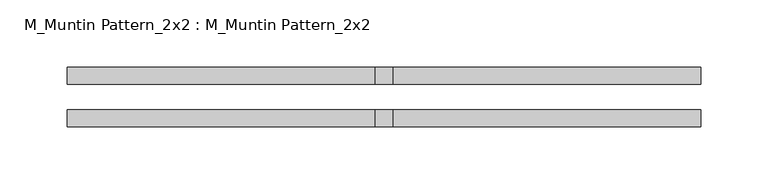
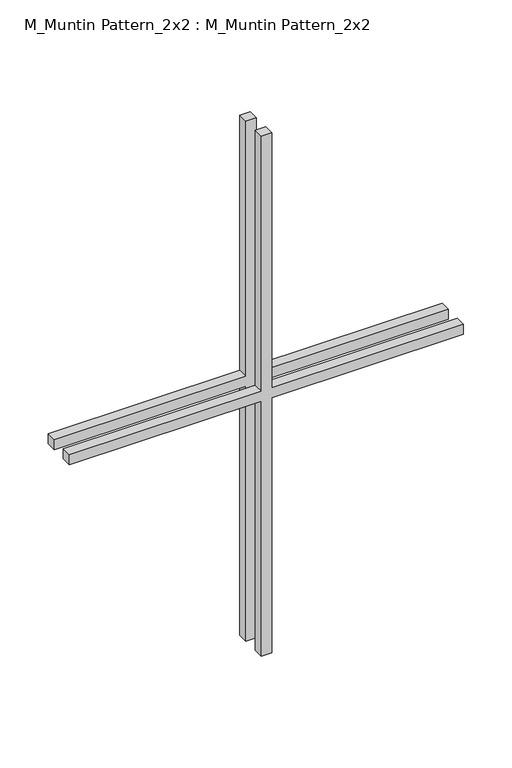
"""IFC4 building model written with IfcOpenShell, lengths in millimetres: proxy geometry, M_Muntin Pattern_2x2 : M_Muntin Pattern_2x2."""

from ifc_helpers import new_model, si_unit, frame, origin, place, context, project, spatial, polyline, outline, extrude, source, transform, mapped, element, save


def m_muntin_pattern_2x2_m_muntin_pattern_2x2_8d9e5da3(model_context):
    return source(origin(), model_context, "Body", "SweptSolid", [
        extrude(outline(polyline([(336.5, -6.35), (336.5, -236.5375), (323.8, -236.5375), (323.8, -6.35), (0.0, -6.35), (0.0, 6.35), (323.8, 6.35), (323.8, 236.5375), (336.5, 236.5375), (336.5, 6.35), (660.3, 6.35), (660.3, -6.35), (336.5, -6.35)])), frame((0.0, 9.525, 0.0), z_axis=(0.0, 1.0, 0.0), x_axis=(0.0, 0.0, 1.0)), (0.0, 0.0, 1.0), 12.7),
        extrude(outline(polyline([(336.5, -6.35), (336.5, -236.5375), (323.8, -236.5375), (323.8, -6.35), (0.0, -6.35), (0.0, 6.35), (323.8, 6.35), (323.8, 236.5375), (336.5, 236.5375), (336.5, 6.35), (660.3, 6.35), (660.3, -6.35), (336.5, -6.35)])), frame((0.0, -22.225, 0.0), z_axis=(0.0, 1.0, 0.0), x_axis=(0.0, 0.0, 1.0)), (0.0, 0.0, 1.0), 12.7),
    ])


if __name__ == "__main__":
    model = new_model("IFC4")
    model_context = context("Model", 3, world=origin())
    ifc_project = project(units=[si_unit("LENGTHUNIT", "METRE", prefix="MILLI")], contexts=[model_context])
    site = spatial("IfcSite", under=ifc_project)
    building = spatial("IfcBuilding", under=site)
    placement = place(None, origin())
    m_muntin_pattern_2x2_m_muntin_pattern_2x2_shape = m_muntin_pattern_2x2_m_muntin_pattern_2x2_8d9e5da3(model_context)
    element("IfcBuildingElementProxy", 1, Name="M_Muntin Pattern_2x2 : M_Muntin Pattern_2x2", ObjectType="M_Muntin Pattern_2x2 : M_Muntin Pattern_2x2", at=placement, inside=building, context=model_context, shape_type="MappedRepresentation", body=[
        mapped(m_muntin_pattern_2x2_m_muntin_pattern_2x2_shape, transform((0.0, 0.0, 0.0), x_axis=(1.0, 0.0, 0.0), y_axis=(0.0, 1.0, 0.0), z_axis=(0.0, 0.0, 1.0))),
    ])
    save(model, "model.ifc")

# Revit data of these elements
# Type "M_Muntin Pattern_2x2 : M_Muntin Pattern_2x2"
#   Width [instance default] = 3' - 11.24409"
#   Thickness = 0' - 0 1/2"
#   Height [instance default] = 3' - 11.24409"
#   Distance = 0' - 0 3/4"
#   Interior Material [instance default] = none
#   Exterior Material [instance default] = none
#   Default Elevation = 0
# Element 1 (IfcBuildingElementProxy, "M_Muntin Pattern_2x2 : M_Muntin Pattern_2x2")
#   Width = 1' - 6 5/8"
#   Height = 2' - 1.99606"
#   Interior Material = Wood - Stained
#   Exterior Material = Clad - White
#   Materials on its faces: "Clad - White", "Wood - Stained"
# Materials
#   "Clad - White": class "Wood", colour RGB 242 242 238, transparency 0, Cost = 0
#   "Wood - Stained": class "Wood", colour RGB 224 178 126, transparency 0, Cost = 0
